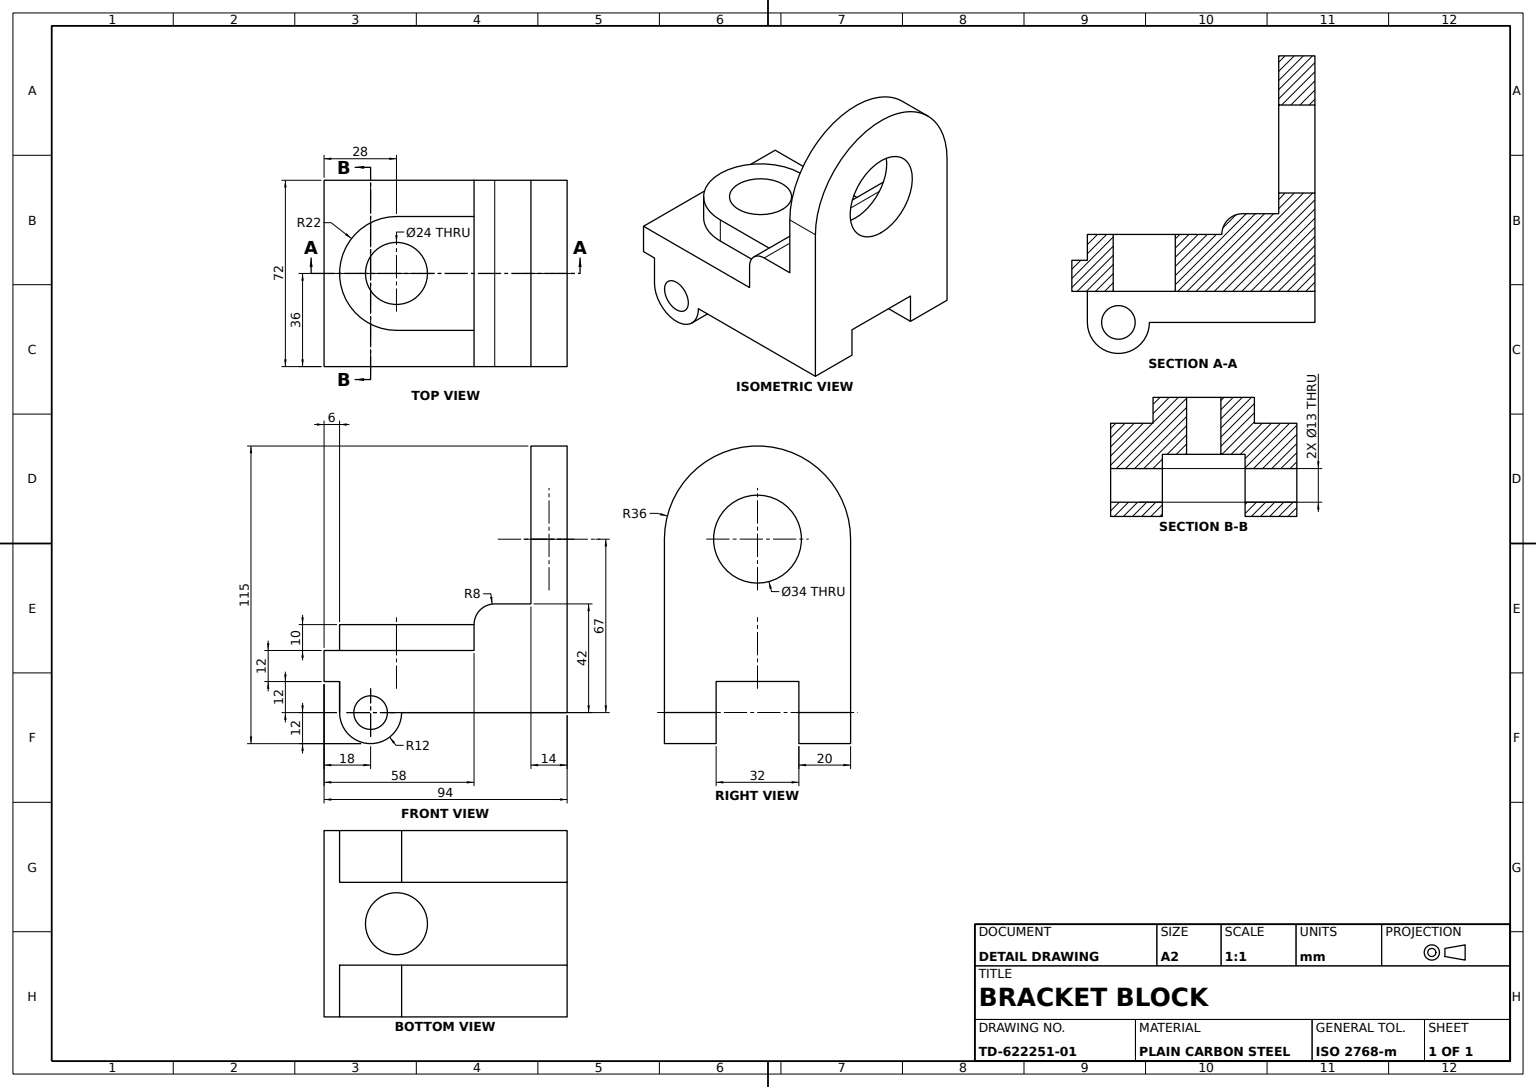
SolidWorks part; units mm, degrees
material "Plain Carbon Steel"
ref_plane "Front Plane" through (0, 0, 0) normal (0, 0, 1) x (1, 0, 0)
ref_plane "Top Plane" through (0, 0, 0) normal (0, 1, 0) x (1, 0, 0)
ref_plane "Right Plane" through (0, 0, 0) normal (1, 0, 0) x (0, 0, -1)
sketch "Base Body Profile" plane through (0, 0, 0) normal (0, 0, 1) x (1, 0, 0)
  line L0 (0, 0) -> (0, 55)
  line L1 (0, 55) -> (-14, 55)
  line L2 (-14, 55) -> (-14, 30)
  line L3 (-14, 30) -> (-28, 30)
  line L4 (-36, 22) -> (-36, 12)
  line L5 (-36, 12) -> (-94, 12)
  line L6 (-94, 12) -> (-94, 0)
  line L7 (-94, 0) -> (-88, 0)
  line L8 (-88, 0) -> (-88, -12)
  line L9 (-64, -12) -> (0, -12)
  line L10 (0, -12) -> (0, 0)
  arc A0 (-28, 30) -> (-36, 22) centre (-28, 22) ccw
  arc A1 (-88, -12) -> (-64, -12) centre (-76, -12) ccw
  circle A2 centre (-76, -12) radius 6.5
  dimension "D1" = 8
  dimension "D6" = 58
  dimension "D11" = 13
  dimension "D2" = 12
  dimension "D3" = 12
  dimension "D4" = 6
  dimension "D5" = 12
  dimension "D7" = 22
  dimension "D8" = 14
  dimension "D9" = 67
  dimension "D10" = 42
extrude "Base Body" add sketch "Base Body Profile" along normal mid plane 72
sketch "Pocket 32x20 Sketch" plane through (-88, 0, 0) normal (-1, 0, 0) x (0, 0, 1)
  line L0 (36, 0) -> (-36, 0) construction
  line L1 (-16, 0) -> (16, 0)
  line L2 (-16, 0) -> (-16, -24)
  line L3 (-16, -24) -> (16, -24)
  line L4 (16, 0) -> (16, -24)
  line L5 (-36, 0) -> (-36, -12) construction
  line L7 (-36, -24) -> (36, -24) construction
  dimension "D1" = 32
  dimension "D2" = 20
extrude "Pocket 32x20" cut sketch "Pocket 32x20 Sketch" against normal through all
sketch "Lug Rounded Top Sketch" plane through (0, 0, 0) normal (1, 0, 0) x (0, 0, -1)
  line L0 (-36, 55) -> (36, 55) construction
  line L1 (-36, -12) -> (-36, 55) construction
  line L2 (-36, 55) -> (36, 55)
  arc A0 (36, 55) -> (-36, 55) centre (0, 55) ccw
extrude "Lug Rounded Top" add sketch "Lug Rounded Top Sketch" against normal up to surface (14 mm away) up to face at (-14, 42.5, 0)
sketch "Lug Bore Sketch" plane through (-14, 0, 0) normal (-1, 0, 0) x (0, 0, 1)
  circle A0 centre (0, 55) radius 17
  arc A1 (36, 55) -> (-36, 55) centre (0, 55) ccw construction
  dimension "D1" = 34
extrude "Lug Bore Ø34" cut sketch "Lug Bore Sketch" against normal up to next
sketch "Boss Profile 44x30" plane through (0, 12, 0) normal (0, 1, 0) x (1, 0, 0)
  line L0 (-66, 22) -> (-36, 22)
  line L1 (-36, -36) -> (-36, 36) construction
  line L2 (-66, -22) -> (-36, -22)
  line L3 (-36, -22) -> (-36, 22)
  arc A0 (-66, 22) -> (-66, -22) centre (-66, 0) ccw
  dimension "D1" = 44
  dimension "D2" = 30
extrude "Boss 10mm" add sketch "Boss Profile 44x30" along normal blind 10
sketch "Boss Bore Sketch" plane through (0, 22, 0) normal (0, 1, 0) x (1, 0, 0)
  circle A0 centre (-66, 0) radius 12
  arc A1 (-66, 22) -> (-66, -22) centre (-66, 0) ccw construction
  dimension "D1" = 24
extrude "Boss Bore Ø24" cut sketch "Boss Bore Sketch" against normal through all
